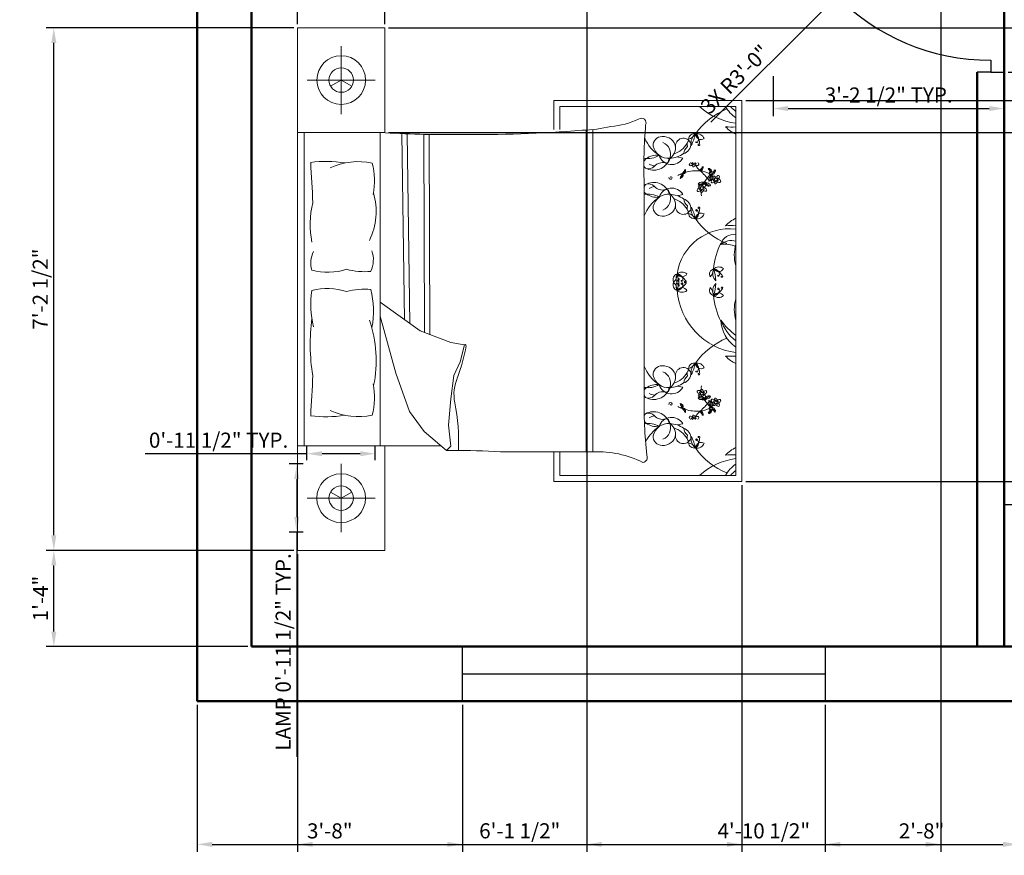
# Model space of a CAD drawing. Units: inches. Extents: x 3242 to 3618, y 1365 to 1814.
# Tile 1 of 6: x 3242 to 3405, y 1376 to 1514. Entities that reach past the tile are written whole.
import ezdxf

# ---------------------------------------------------------------- set-up
doc = ezdxf.new("R2010")
doc.units = ezdxf.units.IN
for name, color, linetype, lineweight in [('A-ANNO-DIMS', 2, 'Continuous', 18), ('A-DOOR', 4, 'Continuous', 25), ('A-FLOR-CASE', 8, 'Continuous', 25), ('A-FURN', 8, 'Continuous', 18), ('A-GLAZ', 5, 'Continuous', 25), ('A-WALL', 7, 'Continuous', 50)]:
    doc.layers.add(name, color=color, linetype=linetype, lineweight=lineweight)
doc.styles.get("Standard").update_dxf_attribs({"font": 'arial.ttf'})
doc.dimstyles.new('ISO-25', dxfattribs={"dimtxt": 2.5, "dimasz": 2.5, "dimexe": 1.25, "dimexo": 0.625, "dimtad": 1, "dimdec": 0, "dimlunit": 3, "dimtxsty": 'Standard', "dimcen": 2.5, "dimadec": 0, "dimazin": 0, "dimtfac": 1, "dimtdec": 0, "dimtmove": 0, "dimatfit": 3, "dimfxl": 1, "dimarcsym": 0})

# ---------------------------------------------------------------- blocks, each defined once
blk = doc.blocks.new('DOOR-SWING-36IN')
for p, q in [((33.75, 40), (38.25, 40)), ((36, 40), (36, 38)), ((36, 38), (0, 38)), ((38.25, 37), (0, 37)), ((36, 2), (36, 0)), ((36, 0), (33.75, 0)), ((36, 0), (38.25, 0))]:
    blk.add_line(p, q)
blk.add_arc((36, 38), 36, 180, 270)
blk = doc.blocks.new('WINDOW-60IN')
for p, q in [((0, 9), (60, 9)), ((0, 0), (0, 9)), ((60, 9), (60, 0)), ((0, 4.5), (60, 4.5)), ((60, 0), (0, 0))]:
    blk.add_line(p, q)
blk = doc.blocks.new('BEDSIDE-LAMP-LG')
for p, q in [((5.65, 0), (5.65, 11.29)), ((11.29, 5.65), (0, 5.65))]:
    blk.add_line(p, q)
for points in [[(5.65, 5.65), (3.9, 4.64)], [(5.65, 5.65), (7.39, 4.64)]]:
    blk.add_lwpolyline(points)
for radius in [4.03, 2.02]:
    blk.add_circle((5.65, 5.65), radius)
blk = doc.blocks.new('*D17')
at = {"layer": 'A-ANNO-DIMS', "color": 0, "lineweight": -2, "transparency": 16777216}
for p, q in [((3405.61, 1545.66), (3412.23, 1545.66)), ((3410.98, 1508.16), (3410.98, 1543.16)), ((3405.61, 1505.66), (3412.23, 1505.66))]:
    blk.add_line(p, q, dxfattribs=at)
at = {"layer": 'A-ANNO-DIMS', "color": 0, "transparency": 16777216}
for points in [[(3410.56, 1543.16), (3411.4, 1543.16), (3410.98, 1545.66)], [(3410.56, 1508.16), (3411.4, 1508.16), (3410.98, 1505.66)]]:
    blk.add_solid(points, dxfattribs=at)
at = {"layer": 'Defpoints', "color": 0, "transparency": 16777216}
for p in [(3404.98, 1545.66), (3410.98, 1545.66), (3404.98, 1505.66)]:
    blk.add_point(p, dxfattribs=at)
at = {"layer": 'A-ANNO-DIMS', "color": 0, "transparency": 16777216, "insert": (3409.06, 1525.66), "char_height": 2.5, "attachment_point": 5, "rotation": 90}
blk.add_mtext('DOOR 3\'-4" TYP.', dxfattribs=at)
blk = doc.blocks.new('*D18')
at = {"layer": 'A-ANNO-DIMS', "color": 0, "lineweight": -2, "transparency": 16777216}
for p, q in [((3366.73, 1505.03), (3366.73, 1498.41)), ((3404.98, 1505.03), (3404.98, 1498.41)), ((3369.23, 1499.66), (3402.48, 1499.66))]:
    blk.add_line(p, q, dxfattribs=at)
at = {"layer": 'A-ANNO-DIMS', "color": 0, "transparency": 16777216}
for points in [[(3369.23, 1500.07), (3369.23, 1499.24), (3366.73, 1499.66)], [(3402.48, 1500.07), (3402.48, 1499.24), (3404.98, 1499.66)]]:
    blk.add_solid(points, dxfattribs=at)
at = {"layer": 'Defpoints', "color": 0, "transparency": 16777216}
for p in [(3366.73, 1505.66), (3404.98, 1505.66), (3404.98, 1499.66)]:
    blk.add_point(p, dxfattribs=at)
at = {"layer": 'A-ANNO-DIMS', "color": 0, "transparency": 16777216, "insert": (3385.86, 1501.57), "char_height": 2.5, "attachment_point": 5}
blk.add_mtext('3\'-2 1/2" TYP.', dxfattribs=at)
blk = doc.blocks.new('*D31')
at = {"layer": 'A-ANNO-DIMS', "color": 0, "lineweight": -2, "transparency": 16777216}
for p, q in [((3289.03, 1440.87), (3286.71, 1440.87)), ((3287.96, 1438.37), (3287.96, 1432.08)), ((3289.03, 1429.58), (3286.71, 1429.58)), ((3287.96, 1429.58), (3287.96, 1392.45))]:
    blk.add_line(p, q, dxfattribs=at)
at = {"layer": 'A-ANNO-DIMS', "color": 0, "transparency": 16777216}
for points in [[(3287.54, 1438.37), (3288.38, 1438.37), (3287.96, 1440.87)], [(3287.54, 1432.08), (3288.38, 1432.08), (3287.96, 1429.58)]]:
    blk.add_solid(points, dxfattribs=at)
at = {"layer": 'Defpoints', "color": 0, "transparency": 16777216}
for p in [(3289.65, 1440.87), (3287.96, 1429.58), (3289.65, 1429.58)]:
    blk.add_point(p, dxfattribs=at)
at = {"layer": 'A-ANNO-DIMS', "color": 0, "transparency": 16777216, "insert": (3286.04, 1409.77), "char_height": 2.5, "attachment_point": 5, "rotation": 90}
blk.add_mtext('LAMP 0\'-11 1/2" TYP.', dxfattribs=at)
blk = doc.blocks.new('*D32')
at = {"layer": 'A-ANNO-DIMS', "color": 0, "lineweight": -2, "transparency": 16777216}
for p, q in [((3289.65, 1441.5), (3289.65, 1443.81)), ((3300.95, 1441.5), (3300.95, 1443.81)), ((3289.65, 1442.56), (3262.9, 1442.56)), ((3298.45, 1442.56), (3292.15, 1442.56))]:
    blk.add_line(p, q, dxfattribs=at)
at = {"layer": 'A-ANNO-DIMS', "color": 0, "transparency": 16777216}
for points in [[(3292.15, 1442.98), (3292.15, 1442.15), (3289.65, 1442.56)], [(3298.45, 1442.98), (3298.45, 1442.15), (3300.95, 1442.56)]]:
    blk.add_solid(points, dxfattribs=at)
at = {"layer": 'Defpoints', "color": 0, "transparency": 16777216}
for p in [(3289.65, 1442.56), (3289.65, 1440.87), (3300.95, 1440.87)]:
    blk.add_point(p, dxfattribs=at)
at = {"layer": 'A-ANNO-DIMS', "color": 0, "transparency": 16777216, "insert": (3275.03, 1444.48), "char_height": 2.5, "attachment_point": 5}
blk.add_mtext('0\'-11 1/2" TYP.', dxfattribs=at)
blk = doc.blocks.new('*D39')
at = {"layer": 'A-ANNO-DIMS', "color": 0, "lineweight": -2, "transparency": 16777216}
for p, q in [((3271.48, 1401.03), (3271.48, 1376.71)), ((3315.35, 1401.03), (3315.35, 1376.71)), ((3273.98, 1377.96), (3312.85, 1377.96))]:
    blk.add_line(p, q, dxfattribs=at)
at = {"layer": 'A-ANNO-DIMS', "color": 0, "transparency": 16777216}
for points in [[(3273.98, 1378.37), (3273.98, 1377.54), (3271.48, 1377.96)], [(3312.85, 1378.37), (3312.85, 1377.54), (3315.35, 1377.96)]]:
    blk.add_solid(points, dxfattribs=at)
at = {"layer": 'Defpoints', "color": 0, "transparency": 16777216}
for p in [(3271.48, 1401.66), (3315.35, 1401.66), (3315.35, 1377.96)]:
    blk.add_point(p, dxfattribs=at)
at = {"layer": 'A-ANNO-DIMS', "color": 0, "transparency": 16777216, "insert": (3293.42, 1379.86), "char_height": 2.5, "attachment_point": 5}
blk.add_mtext('3\'-8"', dxfattribs=at)
blk = doc.blocks.new('*D40')
at = {"layer": 'A-ANNO-DIMS', "color": 0, "lineweight": -2, "transparency": 16777216}
for p, q in [((3375.35, 1401.03), (3375.35, 1376.71)), ((3407.26, 1401.03), (3407.26, 1376.71)), ((3377.85, 1377.96), (3404.76, 1377.96))]:
    blk.add_line(p, q, dxfattribs=at)
at = {"layer": 'A-ANNO-DIMS', "color": 0, "transparency": 16777216}
for points in [[(3377.85, 1378.37), (3377.85, 1377.54), (3375.35, 1377.96)], [(3404.76, 1378.37), (3404.76, 1377.54), (3407.26, 1377.96)]]:
    blk.add_solid(points, dxfattribs=at)
at = {"layer": 'Defpoints', "color": 0, "transparency": 16777216}
for p in [(3375.35, 1401.66), (3407.26, 1401.66), (3407.26, 1377.96)]:
    blk.add_point(p, dxfattribs=at)
at = {"layer": 'A-ANNO-DIMS', "color": 0, "transparency": 16777216, "insert": (3391.3, 1379.86), "char_height": 2.5, "attachment_point": 5}
blk.add_mtext('2\'-8"', dxfattribs=at)
blk = doc.blocks.new('*D48')
at = {"layer": 'A-ANNO-DIMS', "color": 0, "lineweight": -2, "transparency": 16777216}
for p, q in [((3394.48, 1651.75), (3394.48, 1376.71)), ((3335.91, 1642.66), (3335.91, 1376.71)), ((3338.41, 1377.96), (3391.98, 1377.96))]:
    blk.add_line(p, q, dxfattribs=at)
at = {"layer": 'A-ANNO-DIMS', "color": 0, "transparency": 16777216}
for points in [[(3338.41, 1378.37), (3338.41, 1377.54), (3335.91, 1377.96)], [(3391.98, 1378.37), (3391.98, 1377.54), (3394.48, 1377.96)]]:
    blk.add_solid(points, dxfattribs=at)
at = {"layer": 'Defpoints', "color": 0, "transparency": 16777216}
for p in [(3394.48, 1652.37), (3335.91, 1643.28), (3394.48, 1377.96)]:
    blk.add_point(p, dxfattribs=at)
at = {"layer": 'A-ANNO-DIMS', "color": 0, "transparency": 16777216, "insert": (3365.2, 1379.87), "char_height": 2.5, "attachment_point": 5}
blk.add_mtext('4\'-10 1/2"', dxfattribs=at)
blk = doc.blocks.new('*D53')
at = {"layer": 'A-ANNO-DIMS', "color": 0, "lineweight": -2, "transparency": 16777216}
for p, q in [((3361.59, 1437.36), (3361.59, 1376.71)), ((3288.1, 1425.96), (3288.1, 1376.71)), ((3290.6, 1377.96), (3359.09, 1377.96))]:
    blk.add_line(p, q, dxfattribs=at)
at = {"layer": 'A-ANNO-DIMS', "color": 0, "transparency": 16777216}
for points in [[(3290.6, 1378.37), (3290.6, 1377.54), (3288.1, 1377.96)], [(3359.09, 1378.37), (3359.09, 1377.54), (3361.59, 1377.96)]]:
    blk.add_solid(points, dxfattribs=at)
at = {"layer": 'Defpoints', "color": 0, "transparency": 16777216}
for p in [(3361.59, 1437.99), (3288.1, 1426.58), (3361.59, 1377.96)]:
    blk.add_point(p, dxfattribs=at)
at = {"layer": 'A-ANNO-DIMS', "color": 0, "transparency": 16777216, "insert": (3324.84, 1379.87), "char_height": 2.5, "attachment_point": 5}
blk.add_mtext('6\'-1 1/2"', dxfattribs=at)
blk = doc.blocks.new('*D54')
at = {"layer": 'A-ANNO-DIMS', "color": 0, "lineweight": -2, "transparency": 16777216}
for p, q in [((3362.21, 1500.99), (3617.43, 1500.99)), ((3616.18, 1440.49), (3616.18, 1498.49)), ((3362.21, 1437.99), (3617.43, 1437.99))]:
    blk.add_line(p, q, dxfattribs=at)
at = {"layer": 'A-ANNO-DIMS', "color": 0, "transparency": 16777216}
for points in [[(3615.76, 1498.49), (3616.6, 1498.49), (3616.18, 1500.99)], [(3615.76, 1440.49), (3616.6, 1440.49), (3616.18, 1437.99)]]:
    blk.add_solid(points, dxfattribs=at)
at = {"layer": 'Defpoints', "color": 0, "transparency": 16777216}
for p in [(3361.59, 1500.99), (3616.18, 1500.99), (3361.59, 1437.99)]:
    blk.add_point(p, dxfattribs=at)
at = {"layer": 'A-ANNO-DIMS', "color": 0, "transparency": 16777216, "insert": (3614.28, 1469.49), "char_height": 2.5, "attachment_point": 5, "rotation": 90}
blk.add_mtext('5\'-3"', dxfattribs=at)
blk = doc.blocks.new('*D55')
at = {"layer": 'A-ANNO-DIMS', "color": 0, "lineweight": -2, "transparency": 16777216}
for p, q in [((3303.13, 1513), (3617.43, 1513)), ((3616.18, 1510.5), (3616.18, 1498.21)), ((3303.13, 1495.71), (3617.43, 1495.71))]:
    blk.add_line(p, q, dxfattribs=at)
at = {"layer": 'A-ANNO-DIMS', "color": 0, "transparency": 16777216}
for points in [[(3615.76, 1510.5), (3616.6, 1510.5), (3616.18, 1513)], [(3615.76, 1498.21), (3616.6, 1498.21), (3616.18, 1495.71)]]:
    blk.add_solid(points, dxfattribs=at)
at = {"layer": 'Defpoints', "color": 0, "transparency": 16777216}
for p in [(3302.5, 1513), (3302.5, 1495.71), (3616.18, 1495.71)]:
    blk.add_point(p, dxfattribs=at)
at = {"layer": 'A-ANNO-DIMS', "color": 0, "transparency": 16777216, "insert": (3614.26, 1504.35), "char_height": 2.5, "attachment_point": 5, "rotation": 90}
blk.add_mtext('1\'-5 1/2"', dxfattribs=at)
blk = doc.blocks.new('*D56')
at = {"layer": 'A-ANNO-DIMS', "color": 0, "lineweight": -2, "transparency": 16777216}
for p, q in [((3288.1, 1513.62), (3288.1, 1783.61)), ((3302.5, 1513.62), (3302.5, 1783.61)), ((3290.6, 1782.36), (3300, 1782.36))]:
    blk.add_line(p, q, dxfattribs=at)
at = {"layer": 'A-ANNO-DIMS', "color": 0, "transparency": 16777216}
for points in [[(3290.6, 1782.77), (3290.6, 1781.94), (3288.1, 1782.36)], [(3300, 1782.77), (3300, 1781.94), (3302.5, 1782.36)]]:
    blk.add_solid(points, dxfattribs=at)
at = {"layer": 'Defpoints', "color": 0, "transparency": 16777216}
for p in [(3302.5, 1782.36), (3288.1, 1513), (3302.5, 1513)]:
    blk.add_point(p, dxfattribs=at)
at = {"layer": 'A-ANNO-DIMS', "color": 0, "transparency": 16777216, "insert": (3295.3, 1784.27), "char_height": 2.5, "attachment_point": 5}
blk.add_mtext('1\'-2 1/2"', dxfattribs=at)
blk = doc.blocks.new('*D57')
at = {"layer": 'A-ANNO-DIMS', "color": 0, "lineweight": -2, "transparency": 16777216}
for p, q in [((3287.47, 1513), (3246.53, 1513)), ((3247.78, 1429.08), (3247.78, 1510.5)), ((3287.47, 1426.58), (3246.53, 1426.58))]:
    blk.add_line(p, q, dxfattribs=at)
at = {"layer": 'A-ANNO-DIMS', "color": 0, "transparency": 16777216}
for points in [[(3247.36, 1510.5), (3248.2, 1510.5), (3247.78, 1513)], [(3247.36, 1429.08), (3248.2, 1429.08), (3247.78, 1426.58)]]:
    blk.add_solid(points, dxfattribs=at)
at = {"layer": 'Defpoints', "color": 0, "transparency": 16777216}
for p in [(3247.78, 1513), (3288.1, 1513), (3288.1, 1426.58)]:
    blk.add_point(p, dxfattribs=at)
at = {"layer": 'A-ANNO-DIMS', "color": 0, "transparency": 16777216, "insert": (3245.86, 1469.79), "char_height": 2.5, "attachment_point": 5, "rotation": 90}
blk.add_mtext('7\'-2 1/2"', dxfattribs=at)
blk = doc.blocks.new('*D59')
at = {"layer": 'A-ANNO-DIMS', "color": 0, "lineweight": -2, "transparency": 16777216}
for p, q in [((3287.47, 1426.58), (3246.53, 1426.58)), ((3247.78, 1413.16), (3247.78, 1424.08)), ((3279.86, 1410.66), (3246.53, 1410.66))]:
    blk.add_line(p, q, dxfattribs=at)
at = {"layer": 'A-ANNO-DIMS', "color": 0, "transparency": 16777216}
for points in [[(3247.36, 1424.08), (3248.2, 1424.08), (3247.78, 1426.58)], [(3247.36, 1413.16), (3248.2, 1413.16), (3247.78, 1410.66)]]:
    blk.add_solid(points, dxfattribs=at)
at = {"layer": 'Defpoints', "color": 0, "transparency": 16777216}
for p in [(3247.78, 1426.58), (3288.1, 1426.58), (3280.48, 1410.66)]:
    blk.add_point(p, dxfattribs=at)
at = {"layer": 'A-ANNO-DIMS', "color": 0, "transparency": 16777216, "insert": (3245.9, 1418.62), "char_height": 2.5, "attachment_point": 5, "rotation": 90}
blk.add_mtext('1\'-4"', dxfattribs=at)
blk = doc.blocks.new('*D65')
at = {"layer": 'A-ANNO-DIMS', "color": 0, "lineweight": -2, "transparency": 16777216}
for p, q in [((3402.73, 1543.66), (3377.27, 1518.2)), ((3356.46, 1497.39), (3375.51, 1516.43))]:
    blk.add_line(p, q, dxfattribs=at)
at = {"layer": 'A-ANNO-DIMS', "color": 0, "transparency": 16777216}
blk.add_solid([(3375.21, 1516.73), (3375.8, 1516.14), (3377.27, 1518.2)], dxfattribs=at)
at = {"layer": 'Defpoints', "color": 0, "transparency": 16777216}
for p in [(3402.73, 1543.66), (3377.27, 1518.2)]:
    blk.add_point(p, dxfattribs=at)
at = {"layer": 'A-ANNO-DIMS', "color": 0, "transparency": 16777216, "insert": (3360.66, 1504.27), "char_height": 2.5, "attachment_point": 5, "rotation": 44.9992}
blk.add_mtext('3X R3\'-0"', dxfattribs=at)

msp = doc.modelspace()

# ---------------------------------------------------------------- linework, layer by layer
at = {"layer": 'A-FLOR-CASE'}
msp.add_line((3483.26, 1434.12), (3404.98, 1434.12), dxfattribs=at)
at = {"layer": 'A-FURN'}
for p, q in [((3288.1, 1426.58), (3288.1, 1513)), ((3330.46, 1496.2), (3330.46, 1500.99)), ((3330.46, 1500.99), (3361.59, 1500.99)), ((3331.46, 1499.99), (3331.46, 1496.18)), ((3360.59, 1499.99), (3331.46, 1499.99)), ((3360.59, 1438.99), (3360.59, 1499.99)), ((3361.59, 1500.99), (3361.59, 1437.99)), ((3289.21, 1495.71), (3289.21, 1443.87)), ((3301.75, 1443.87), (3301.75, 1495.71)), ((3305.34, 1495.48), (3305.78, 1464.72)), ((3306.23, 1495.45), (3306.67, 1464.07)), ((3308.95, 1495.4), (3309.08, 1462.59)), ((3309.84, 1495.41), (3309.98, 1462.25)), ((3335.85, 1496.11), (3335.85, 1442.87)), ((3336.93, 1496.19), (3336.93, 1442.87)), ((3351.82, 1491.47), (3350.85, 1491.66)), ((3345.41, 1487.33), (3345.41, 1452.25)), ((3351.82, 1485.43), (3350.85, 1485.24)), ((3301.75, 1467.61), (3308.35, 1462.87)), ((3304.32, 1455.87), (3301.75, 1465.29)), ((3308.35, 1462.87), (3313.42, 1460.94)), ((3313.42, 1460.94), (3315.69, 1460.59)), ((3315.69, 1460.59), (3314.99, 1457.79)), ((3314.99, 1457.79), (3313.94, 1455.52)), ((3306.6, 1449.57), (3304.32, 1455.87)), ((3313.94, 1455.52), (3313.42, 1451.67)), ((3351.82, 1453.55), (3350.85, 1453.74)), ((3313.42, 1451.67), (3313.07, 1447.29)), ((3309.05, 1446.24), (3306.6, 1449.57)), ((3312.72, 1443.09), (3309.05, 1446.24)), ((3313.07, 1447.29), (3313.42, 1443.79)), ((3351.82, 1447.51), (3350.85, 1447.32)), ((3288.1, 1443.87), (3311.82, 1443.87)), ((3313.42, 1443.79), (3312.72, 1443.09)), ((3330.46, 1437.99), (3330.46, 1442.88)), ((3331.46, 1442.88), (3331.46, 1438.99)), ((3361.59, 1437.99), (3330.46, 1437.99)), ((3331.46, 1438.99), (3360.59, 1438.99))]:
    msp.add_line(p, q, dxfattribs=at)
for points in [[(3288.1, 1495.71), (3302.5, 1495.71), (3302.5, 1513), (3288.1, 1513)], [(3302.5, 1443.87), (3302.5, 1426.58), (3288.1, 1426.58)]]:
    msp.add_lwpolyline(points, dxfattribs=at)
for points in [[(3335.17, 1496.08, 0.056112), (3339.92, 1496.71, 0.095341), (3344.5, 1497.92)], [(3290.25, 1490.75, -0.074897), (3295.9, 1490.65, 0.472817)], [(3296.21, 1473.08, -0.14099), (3290.45, 1472.9, -0.235245)], [(3296.21, 1469.38, 0.14099), (3290.45, 1469.56, 0.235245)], [(3290.25, 1448.83, 0.074897), (3295.9, 1448.93, -0.472817)], [(3320.63, 1442.91, 0.001242), (3337.03, 1442.87, -0.127202), (3345.2, 1441.14)]]:
    msp.add_lwpolyline(points, format="xyb", dxfattribs=at)
for centre in [(3357.28, 1487.92), (3354.96, 1486.48), (3354.96, 1452.5), (3357.28, 1451.06)]:
    msp.add_circle(centre, 0.22, dxfattribs=at)
for centre, radius, start, end in [((3362.11, 1508.39), 11.28, 228.1144, 262.255), ((3363.62, 1502.73), 5.5, 209.8884, 236.5383), ((3364.64, 1504.7), 6.85, 223.5186, 233.6964), ((3363.22, 1489.08), 11.28, 111.4092, 145.6135), ((3344.94, 1497.27), 0.788, 336.5219, 123.8264), ((3429.46, 1489.98), 84.09, 175.2402, 181.8035), ((3362.35, 1499.65), 4.59, 221.0454, 247.4453), ((3359.88, 1512.21), 15.61, 266.3481, 272.5919), ((3312.32, 1650.62), 155.27, 266.1, 270.9282), ((3317.96, 1697.89), 202.54, 269.1145, 274.8735), ((3348.36, 1493.57), 1.46, 88.9462, 185.5144), ((3348.57, 1492.97), 2.06, 7.1143, 95.0551), ((3353.69, 1494.55), 0.935, 76.272, 177.0484), ((3352.26, 1496.46), 1.93, 284.7031, 328.6173), ((3354.95, 1494.01), 1.78, 125.7657, 194.5347), ((3346.2, 1497.17), 7.89, 332.8176, 347.4827), ((3354.18, 1494.23), 1.25, 20.9613, 102.2885), ((3354.85, 1495.48), 0.942, 181.7131, 301.5367), ((3351.76, 1493.58), 2.85, 2.0648, 41.1598), ((3353.48, 1494.64), 0.923, 316.2238, 62.3173), ((3351.5, 1497.38), 6.54, 203.6453, 236.3329), ((3349.44, 1494.02), 2.6, 193.079, 274.7067), ((3347.78, 1492.16), 2.01, 338.5779, 68.4181), ((3349.04, 1496.02), 4.08, 288.2955, 328.7386), ((3351.89, 1493.45), 1.3, 19.1312, 189.736), ((3351.5, 1493.76), 1.62, 285.6955, 4.031), ((3353.66, 1492.01), 1.72, 128.4175, 173.8338), ((3353.3, 1493.71), 0.795, 126.7319, 206.0245), ((3354.01, 1494.1), 0.0736, 20.2667, 316.2271), ((3354.47, 1493.67), 0.14, 168.5166, 2.0648), ((3354.4, 1493.69), 0.0681, 52.0591, 168.5166), ((3346.05, 1494.98), 3.58, 259.249, 301.1782), ((3347.61, 1488.62), 3.33, 85.2696, 124.215), ((3349.96, 1492.54), 2.15, 196.8663, 330.0915), ((3348.11, 1493.33), 2.51, 305.9599, 357.6409), ((3349.37, 1496.06), 4.64, 273.4924, 303.7117), ((2467.9, 1443.12), 823.74, 2.85022, 3.31479), ((3298.16, 1479.74), 11.14, 78.2417, 114.8684), ((3289.24, 1487.67), 11.58, 348.9631, 14.8961), ((3346.37, 1490.55), 1.04, 196.6343, 225.5483), ((3346.37, 1490.55), 1.04, 127.675, 162.5814), ((3346.98, 1492.21), 2.75, 240.8249, 340.7178), ((3346.16, 1490.99), 1.29, 246.1646, 318.4347), ((3347.48, 1492.62), 2.48, 240.0851, 262.564), ((3348.46, 1488.95), 1.77, 74.8529, 138.4347), ((3349.06, 1491.18), 0.536, 254.8529, 12.6959), ((3347.61, 1488.62), 3.33, 53.6555, 57.2989), ((3353.05, 1490.37), 0.17, 125.0752, 284.7644), ((3353.31, 1490.44), 0.367, 127.3642, 168.4363), ((3353.02, 1490.73), 0.529, 277.4968, 341.2737), ((3353.44, 1490.49), 0.21, 88.1325, 178.8919), ((3353.86, 1490.26), 0.455, 136.3462, 189.6513), ((3353.6, 1490.22), 0.19, 189.6513, 312.3208), ((3353.65, 1490.74), 0.22, 183.2768, 356.7232), ((3354.34, 1490.35), 0.72, 164.2829, 186.9148), ((3353.49, 1490.35), 0.36, 312.3208, 40.2111), ((3354.25, 1490.75), 0.511, 201.6382, 274.947), ((3353.57, 1490.05), 0.668, 42.3896, 66.5724), ((3360.31, 1495.34), 8.2, 217.9541, 226.8459), ((3354.06, 1490.44), 0.363, 10.9597, 52.2379), ((3354.28, 1490.41), 0.169, 274.947, 37.5263), ((3355.35, 1489.67), 0.454, 115.5379, 168.6744), ((3353.82, 1490.32), 1.37, 329.344, 349.7412), ((3352.72, 1490.01), 2.44, 352.8698, 1.6736), ((3354.22, 1482.21), 7.16, 110.1059, 116.9968), ((3351.82, 1488.11), 0.454, 129.5056, 182.6421), ((3350.52, 1489.16), 1.37, 308.4388, 328.836), ((3350.26, 1489.02), 1.39, 336.3901, 344.4871), ((3351.77, 1488.66), 0.176, 83.9457, 185.6216), ((3351.07, 1488.83), 0.724, 328.836, 0.8141), ((3351.44, 1488.62), 0.415, 306.5232, 32.4668), ((3351.94, 1488.94), 0.176, 112.5583, 214.2343), ((3351.82, 1489.25), 0.415, 265.7131, 351.6568), ((3351.46, 1489.48), 0.724, 297.3659, 329.344), ((3350.91, 1490.11), 1.39, 313.6929, 321.7899), ((3352.45, 1489.16), 0.454, 115.5379, 168.6744), ((3350.91, 1489.81), 1.37, 329.344, 349.7412), ((3354.22, 1482.21), 7.16, 86.1723, 106.4158), ((3349.82, 1489.5), 2.44, 352.8698, 1.6736), ((3354.85, 1489.45), 0.176, 112.5583, 214.2343), ((3354.73, 1489.77), 0.415, 265.7131, 351.6568), ((3354.37, 1490), 0.724, 297.3659, 329.344), ((3354.4, 1485.78), 3.59, 60.7959, 85.244), ((3346.76, 1480.61), 11.81, 37.8256, 47.7588), ((3353.82, 1490.62), 1.39, 313.6929, 321.7899), ((3359.17, 1485.41), 4.3, 130.182, 149.456), ((3356.15, 1489.52), 0.246, 33.0979, 123.1364), ((3350.74, 1486.05), 6.43, 31.1156, 34.8118), ((3355.79, 1489.1), 0.665, 2.3172, 70.5201), ((3355.47, 1488.38), 1, 310.9365, 22.7695), ((3356.34, 1488.93), 0.192, 135.7354, 318.1297), ((3356.02, 1489.25), 0.254, 315.7354, 31.1156), ((3355.81, 1488.71), 0.59, 319.3812, 5.5456), ((3356.49, 1488.93), 0.192, 68.2452, 250.6395), ((3356.05, 1489.17), 0.573, 352.6008, 57.1845), ((3358.09, 1485.33), 3.83, 111.7087, 116.2181), ((3354.4, 1485.78), 3.59, 47.5083, 55.9967), ((3356.59, 1489.3), 0.573, 252.8042, 349.6943), ((3356.05, 1488.28), 0.61, 331.1838, 51.6792), ((3356.65, 1489.35), 0.254, 248.2452, 323.6254), ((3356.43, 1489.5), 0.665, 291.7087, 3.0299), ((3356.97, 1488.16), 0.3, 358.5719, 143.8954), ((3351.68, 1493.01), 6.43, 323.6254, 327.3216), ((3356.95, 1489.34), 0.246, 325.6077, 55.6462), ((3357.94, 1487.98), 0.694, 121.9501, 165.2442), ((3357.44, 1488.37), 0.434, 278.5614, 22.5914), ((3357.69, 1488.38), 0.218, 44.3732, 121.9501), ((3346.37, 1486.35), 1.04, 134.4517, 156.7144), ((3346.98, 1484.69), 2.75, 19.2822, 119.1751), ((3346.16, 1485.91), 1.29, 41.5653, 113.8354), ((3349.77, 1488.22), 0.271, 169.5864, 349.5616), ((3349.87, 1488.2), 0.167, 349.5616, 167.2949), ((3350.28, 1490.27), 2.44, 296.5064, 305.3102), ((3354.63, 1488.16), 1, 253.6301, 325.4631), ((3354.91, 1486.77), 0.71, 82.0748, 142.6895), ((3354.83, 1487.75), 0.729, 228.342, 274.9894), ((3354.57, 1486.75), 0.216, 138.2946, 276.2474), ((3354.65, 1486.72), 0.3, 358.5719, 143.8954), ((3354.82, 1486.96), 0.303, 208.8493, 269.9355), ((3354.85, 1487.63), 0.61, 273.8774, 357.1501), ((3355.62, 1486.54), 0.694, 121.9501, 165.2442), ((3355.09, 1488.06), 0.59, 262.0748, 308.2393), ((3355.14, 1486.8), 0.146, 262.868, 7.094), ((3355.12, 1486.93), 0.434, 278.5614, 22.5914), ((3359.17, 1485.41), 4.3, 156.1523, 156.9499), ((3355.37, 1486.94), 0.218, 44.3732, 121.9501), ((3356.04, 1487.45), 0.61, 181.4625, 249.4747), ((3355.94, 1487.93), 0.59, 215.1128, 261.2773), ((3356.41, 1487.9), 1, 197.889, 269.722), ((3356.1, 1487.56), 0.729, 248.3627, 295.0101), ((3355.74, 1486.65), 0.71, 20.6625, 81.2773), ((3356.8, 1487.86), 0.71, 139.3812, 199.9959), ((3355.94, 1488.32), 0.729, 285.6484, 332.2957), ((3356.67, 1487.55), 0.17, 125.0752, 284.7644), ((3356.93, 1487.61), 0.367, 93.635, 168.4363), ((3356.89, 1488.19), 0.216, 138.2946, 276.2474), ((3356.65, 1487.91), 0.529, 277.4968, 341.2737), ((3357.07, 1487.66), 0.21, 88.1325, 178.8919), ((3357.14, 1488.4), 0.303, 208.8493, 269.9355), ((3356.89, 1488.32), 0.346, 274.2123, 318.1587), ((3357.49, 1487.44), 0.455, 136.3462, 189.6513), ((3357.23, 1487.39), 0.19, 189.6513, 312.3208), ((3357.96, 1487.52), 0.72, 164.2829, 186.9148), ((3357.11, 1487.52), 0.36, 312.3208, 40.2111), ((3357.88, 1487.93), 0.511, 201.6382, 274.947), ((3357.46, 1488.24), 0.146, 262.868, 7.094), ((3357.2, 1487.23), 0.668, 42.3896, 66.5724), ((3357.68, 1487.62), 0.363, 10.9597, 118.7804), ((3357.91, 1487.58), 0.169, 274.947, 37.5263), ((3290.09, 1482.67), 11, 333.8761, 16.1746), ((3346.37, 1486.35), 1.04, 203.2856, 232.325), ((3346.05, 1481.92), 3.58, 58.8218, 100.2867), ((3347.61, 1488.29), 3.33, 235.785, 274.7304), ((3347.48, 1484.28), 2.48, 97.436, 119.9149), ((3349.44, 1482.88), 2.6, 85.2933, 166.921), ((3348.46, 1487.95), 1.77, 221.5653, 285.1471), ((3349.96, 1484.36), 2.15, 29.9085, 163.1337), ((3347.78, 1484.74), 2.01, 291.5819, 21.4221), ((3349.06, 1485.72), 0.536, 347.3041, 105.1471), ((3347.61, 1488.29), 3.33, 302.7011, 306.3445), ((3348.11, 1483.57), 2.51, 2.3591, 54.0401), ((3349.37, 1480.85), 4.64, 56.2883, 86.5076), ((3354.35, 1486.11), 0.17, 125.0752, 284.7644), ((3354.61, 1486.17), 0.367, 93.635, 168.4363), ((3354.33, 1486.47), 0.529, 277.4968, 341.2737), ((3354.75, 1486.22), 0.21, 88.1325, 178.8919), ((3354.57, 1486.89), 0.346, 274.2123, 318.1587), ((3355.17, 1486), 0.455, 136.3462, 189.6513), ((3354.91, 1485.95), 0.19, 189.6513, 312.3208), ((3359.17, 1485.41), 4.3, 175.2415, 182.8929), ((3355.64, 1486.08), 0.72, 164.2829, 186.9148), ((3354.79, 1486.08), 0.36, 312.3208, 40.2111), ((3355.56, 1486.49), 0.511, 201.6382, 274.947), ((3354.88, 1485.79), 0.668, 42.3896, 66.5724), ((3355.36, 1486.18), 0.363, 10.9597, 118.7804), ((3355.59, 1486.14), 0.169, 274.947, 37.5263), ((3305.37, 1480.49), 15.19, 166.3427, 191.1841), ((3351.5, 1479.52), 6.54, 123.6671, 158.5059), ((3348.57, 1483.93), 2.06, 264.9449, 352.8857), ((3349.04, 1480.88), 4.08, 31.2614, 71.7045), ((3351.89, 1483.45), 1.3, 170.264, 340.8688), ((3353.66, 1484.89), 1.72, 186.1662, 231.5825), ((3351.5, 1483.14), 1.62, 355.969, 74.3045), ((3353.3, 1483.19), 0.795, 153.9755, 233.2681), ((3348.36, 1483.33), 1.46, 174.4856, 271.0538), ((3353.69, 1482.36), 0.935, 182.9516, 283.728), ((3352.26, 1480.44), 1.93, 31.3827, 75.2969), ((3354.95, 1482.9), 1.78, 165.4653, 234.2343), ((3346.2, 1479.74), 7.89, 12.5173, 27.1824), ((3351.76, 1483.33), 2.85, 318.8402, 357.9352), ((3353.48, 1482.26), 0.923, 297.6827, 43.7762), ((3354.85, 1481.42), 0.942, 58.4633, 178.2869), ((3354.18, 1482.67), 1.25, 257.7115, 339.0387), ((3354.06, 1482.82), 0.122, 43.7762, 339.7183), ((3354.47, 1483.23), 0.14, 357.9352, 191.4834), ((3354.4, 1483.21), 0.0681, 191.4834, 307.9409), ((3363.22, 1487.82), 11.28, 214.3865, 248.5908), ((3362.35, 1477.26), 4.59, 112.5547, 138.9546), ((3359.88, 1464.69), 15.61, 87.4081, 93.6519), ((3359.5, 1471.03), 8.73, 82.8636, 171.8197), ((3360.11, 1476.79), 2.03, 76.3898, 169.0739), ((3368.15, 1472.26), 11.28, 152.5854, 175.5377), ((3359.83, 1475.27), 2.56, 72.8609, 131.9049), ((3358.7, 1472.16), 5.05, 68.117, 96.6195), ((3366.52, 1475.42), 6.2, 162.9798, 196.4569), ((3294.56, 1474.09), 4.27, 153.3437, 196.1026), ((3296.05, 1474.67), 4.58, 335.0183, 18.5407), ((3369.72, 1472.96), 9.18, 174.3643, 175.6213), ((3299.1, 1483.26), 10.59, 254.1707, 275.9871), ((3351.12, 1471.38), 0.935, 106.1963, 206.9726), ((3348.93, 1472.32), 1.93, 314.6273, 358.5415), ((3352.48, 1471.54), 1.78, 155.6899, 224.4589), ((3351.7, 1471.35), 1.25, 50.8855, 132.2127), ((3351.66, 1472.77), 0.942, 211.6373, 331.4609), ((3350.89, 1471.35), 0.923, 346.148, 92.2415), ((3349.93, 1469.57), 2.85, 31.989, 71.0841), ((3343.32, 1469.91), 7.89, 2.7418, 17.407), ((3357.16, 1472.24), 0.935, 106.1963, 206.9726), ((3354.97, 1473.19), 1.93, 314.6273, 358.5415), ((3358.53, 1472.4), 1.78, 155.6899, 224.4589), ((3357.74, 1472.21), 1.25, 50.8855, 132.2127), ((3357.7, 1473.63), 0.942, 211.6373, 331.4609), ((3355.97, 1470.44), 2.85, 31.989, 71.0841), ((3349.37, 1470.78), 7.89, 2.7418, 17.407), ((3356.94, 1472.21), 0.923, 346.148, 92.2415), ((3376, 1468.12), 16.4, 160.0972, 160.2783), ((3351.12, 1470.48), 0.935, 153.0274, 253.8037), ((3348.93, 1469.53), 1.93, 1.4585, 45.3727), ((3352.48, 1470.32), 1.78, 135.5411, 204.3101), ((3343.32, 1471.95), 7.89, 342.593, 357.2582), ((3349.93, 1472.28), 2.85, 288.9159, 328.011), ((3350.89, 1470.51), 0.923, 267.7585, 13.852), ((3351.62, 1471.15), 0.0736, 50.1909, 346.0209), ((3351.67, 1470.7), 0.122, 13.852, 309.9245), ((3352.23, 1471.01), 0.14, 198.4408, 31.989), ((3352.16, 1470.99), 0.0681, 81.9833, 198.4408), ((3352.23, 1470.85), 0.14, 328.011, 161.5592), ((3352.16, 1470.87), 0.0681, 161.5592, 278.0167), ((3358.53, 1469.45), 1.78, 135.5411, 204.3101), ((3349.37, 1471.08), 7.89, 342.593, 357.2582), ((3357.67, 1472.01), 0.0736, 50.1909, 346.0209), ((3358.28, 1471.88), 0.14, 198.4408, 31.989), ((3358.21, 1471.85), 0.0681, 81.9833, 198.4408), ((3305.68, 1467.29), 15.4, 171.5249, 193.96), ((3299.1, 1459.2), 10.59, 84.0129, 105.8293), ((3285.4, 1466.14), 15.24, 349.8617, 13.6238), ((3351.66, 1469.09), 0.942, 28.5391, 148.3627), ((3351.7, 1470.51), 1.25, 227.7873, 309.1145), ((3362.11, 1470.46), 11.28, 184.4623, 262.255), ((3357.16, 1469.62), 0.935, 153.0274, 253.8037), ((3354.97, 1468.67), 1.93, 1.4585, 45.3727), ((3355.97, 1471.42), 2.85, 288.9159, 328.011), ((3356.94, 1469.64), 0.923, 267.7585, 13.852), ((3357.7, 1468.23), 0.942, 28.5391, 148.3627), ((3357.71, 1469.83), 0.122, 13.852, 309.9245), ((3358.28, 1469.98), 0.14, 328.011, 161.5592), ((3358.21, 1470), 0.0681, 161.5592, 278.0167), ((3357.74, 1469.65), 1.25, 227.7873, 309.1145), ((3368.15, 1469.6), 11.28, 184.4623, 207.4146), ((3366.52, 1466.44), 6.2, 163.5431, 197.0202), ((3369.72, 1468.9), 9.18, 184.3787, 185.6357), ((3376, 1473.73), 16.4, 199.7217, 199.9028), ((3321.52, 1460.67), 31.34, 172.2196, 189.497), ((3281.01, 1458.01), 20.09, 348.0397, 19.2615), ((3363.62, 1464.8), 5.5, 181.272, 236.5383), ((3366.57, 1470.38), 10.19, 214.0123, 234.053), ((3364.64, 1466.78), 6.85, 197.8504, 233.6964), ((3363.22, 1451.16), 11.28, 111.4092, 145.6135), ((3283.04, 1466.59), 33.51, 340.1194, 349.3383), ((3315.76, 1460.4), 0.209, 358.8623, 109.7536), ((3353.69, 1456.62), 0.935, 76.272, 177.0484), ((3352.26, 1458.53), 1.93, 284.7031, 328.6173), ((3354.95, 1456.08), 1.78, 125.7657, 194.5347), ((3346.2, 1459.24), 7.89, 332.8176, 347.4827), ((3354.18, 1456.31), 1.25, 20.9613, 102.2885), ((3353.48, 1456.71), 0.923, 316.2238, 62.3173), ((3351.76, 1455.65), 2.85, 2.0648, 41.1598), ((3354.85, 1457.56), 0.942, 181.7131, 301.5367), ((3359.88, 1474.29), 15.61, 266.3481, 272.5919), ((3362.35, 1461.72), 4.59, 221.0454, 247.4453), ((3351.5, 1459.45), 6.54, 201.4941, 236.3329), ((3348.36, 1455.65), 1.46, 88.9462, 185.5144), ((3348.57, 1455.05), 2.06, 7.1143, 95.0551), ((3347.78, 1454.24), 2.01, 338.5779, 68.4181), ((3349.04, 1458.09), 4.08, 288.2955, 328.7386), ((3351.89, 1455.52), 1.3, 19.1312, 189.736), ((3351.5, 1455.83), 1.62, 285.6955, 4.031), ((3353.3, 1455.79), 0.795, 126.7319, 206.0245), ((3354.01, 1456.17), 0.0736, 20.2667, 316.2271), ((2467.9, 1496.46), 823.74, 356.68521, 357.14978), ((3320.99, 1452.37), 7.03, 156.2616, 191.3392), ((3349.44, 1456.09), 2.6, 193.079, 274.7067), ((3348.11, 1455.41), 2.51, 305.9599, 357.6409), ((3349.37, 1458.13), 4.64, 273.4924, 303.7117), ((3353.66, 1454.09), 1.72, 128.4175, 173.8338), ((3354.47, 1455.75), 0.14, 168.5166, 2.0648), ((3354.4, 1455.76), 0.0681, 52.0591, 168.5166), ((3289.24, 1451.91), 11.58, 345.1039, 11.0369), ((3346.05, 1457.06), 3.58, 259.7133, 301.1782), ((3346.37, 1452.62), 1.04, 127.675, 156.7144), ((3346.98, 1454.28), 2.75, 240.8249, 340.7178), ((3347.61, 1450.69), 3.33, 85.2696, 124.215), ((3348.46, 1451.03), 1.77, 74.8529, 138.4347), ((3349.96, 1454.62), 2.15, 196.8663, 330.0915), ((3349.06, 1453.26), 0.536, 254.8529, 12.6959), ((3347.61, 1450.69), 3.33, 53.6555, 57.2989), ((3354.35, 1452.87), 0.17, 75.2356, 234.9248), ((3354.61, 1452.8), 0.367, 191.5637, 266.365), ((3354.33, 1452.51), 0.529, 18.7263, 82.5032), ((3354.75, 1452.75), 0.21, 181.1081, 271.8675), ((3354.91, 1453.02), 0.19, 47.6792, 170.3487), ((3355.17, 1452.98), 0.455, 170.3487, 223.6538), ((3359.17, 1453.57), 4.3, 177.1071, 184.7585), ((3355.64, 1452.89), 0.72, 173.0852, 195.7171), ((3354.79, 1452.9), 0.36, 319.7889, 47.6792), ((3355.56, 1452.49), 0.511, 85.053, 158.3618), ((3354.88, 1453.19), 0.668, 293.4276, 317.6104), ((3355.36, 1452.8), 0.363, 241.2196, 349.0403), ((3355.59, 1452.83), 0.169, 322.4737, 85.053), ((3282.12, 1444.57), 32.61, 357.4519, 11.3392), ((3435.36, 1451.22), 89.96, 179.3433, 185.6887), ((3346.37, 1452.62), 1.04, 203.229, 225.5483), ((3346.16, 1453.06), 1.29, 246.1646, 318.4347), ((3347.48, 1454.7), 2.48, 240.0851, 262.564), ((3349.77, 1450.75), 0.271, 10.4384, 190.4136), ((3354.57, 1452.22), 0.216, 83.7526, 221.7054), ((3354.83, 1451.23), 0.729, 85.0106, 131.658), ((3354.63, 1450.81), 1, 34.5369, 106.3699), ((3354.91, 1452.21), 0.71, 217.3105, 277.9252), ((3354.65, 1452.26), 0.3, 216.1046, 1.4281), ((3354.82, 1452.02), 0.303, 90.0645, 151.1507), ((3354.57, 1452.09), 0.346, 41.8413, 85.7877), ((3346.76, 1458.36), 11.81, 312.2412, 322.1744), ((3354.85, 1451.35), 0.61, 2.8499, 86.1226), ((3355.62, 1452.44), 0.694, 194.7558, 238.0499), ((3355.09, 1450.92), 0.59, 51.7607, 97.9252), ((3355.14, 1452.17), 0.146, 352.906, 97.132), ((3355.12, 1452.05), 0.434, 337.4086, 81.4386), ((3359.17, 1453.57), 4.3, 203.0501, 203.8477), ((3355.37, 1452.04), 0.218, 238.0499, 315.6268), ((3356.04, 1451.52), 0.61, 110.5253, 178.5375), ((3356.41, 1451.07), 1, 90.278, 162.111), ((3355.94, 1451.04), 0.59, 98.7227, 144.8872), ((3359.17, 1453.57), 4.3, 210.544, 229.818), ((3356.1, 1451.42), 0.729, 64.9899, 111.6373), ((3355.74, 1452.33), 0.71, 278.7227, 339.3375), ((3356.8, 1451.12), 0.71, 160.0041, 220.6188), ((3355.47, 1450.6), 1, 337.2305, 49.0635), ((3355.94, 1450.66), 0.729, 27.7043, 74.3516), ((3356.05, 1450.7), 0.61, 308.3208, 28.8162), ((3356.67, 1451.43), 0.17, 75.2356, 234.9248), ((3356.93, 1451.36), 0.367, 191.5637, 266.365), ((3356.89, 1450.78), 0.216, 83.7526, 221.7054), ((3356.65, 1451.07), 0.529, 18.7263, 82.5032), ((3357.07, 1451.32), 0.21, 181.1081, 271.8675), ((3356.89, 1450.65), 0.346, 41.8413, 85.7877), ((3357.23, 1451.58), 0.19, 47.6792, 170.3487), ((3357.49, 1451.54), 0.455, 170.3487, 223.6538), ((3357.96, 1451.45), 0.72, 173.0852, 195.7171), ((3357.11, 1451.46), 0.36, 319.7889, 47.6792), ((3357.88, 1451.05), 0.511, 85.053, 158.3618), ((3357.2, 1451.75), 0.668, 293.4276, 317.6104), ((3357.68, 1451.36), 0.363, 241.2196, 349.0403), ((3357.44, 1450.61), 0.434, 337.4086, 81.4386), ((3357.91, 1451.39), 0.169, 322.4737, 85.053), ((3298.16, 1459.84), 11.14, 245.1316, 281.7583), ((3346.98, 1446.77), 2.75, 19.2822, 119.1751), ((3349.87, 1450.77), 0.167, 192.7051, 10.4384), ((3354.22, 1456.76), 7.16, 243.0032, 249.8941), ((3350.52, 1449.82), 1.37, 31.164, 51.5612), ((3351.82, 1450.86), 0.454, 177.3579, 230.4944), ((3350.28, 1448.7), 2.44, 54.6898, 63.4936), ((3350.26, 1449.96), 1.39, 15.5129, 23.6099), ((3351.77, 1450.31), 0.176, 174.3784, 276.0543), ((3351.44, 1450.36), 0.415, 327.5332, 53.4768), ((3351.07, 1450.15), 0.724, 359.1859, 31.164), ((3351.94, 1450.04), 0.176, 145.7657, 247.4417), ((3351.82, 1449.72), 0.415, 8.3432, 94.2869), ((3351.46, 1449.49), 0.724, 30.656, 62.6341), ((3350.91, 1448.87), 1.39, 38.2101, 46.3071), ((3352.45, 1449.82), 0.454, 191.3256, 244.4621), ((3350.91, 1449.17), 1.37, 10.2588, 30.656), ((3354.22, 1456.76), 7.16, 253.5842, 273.8277), ((3349.82, 1449.48), 2.44, 358.3264, 7.1302), ((3360.31, 1443.64), 8.2, 133.1541, 142.0459), ((3354.85, 1449.52), 0.176, 145.7657, 247.4417), ((3354.4, 1453.2), 3.59, 274.756, 299.2041), ((3354.73, 1449.21), 0.415, 8.3432, 94.2869), ((3354.37, 1448.98), 0.724, 30.656, 62.6341), ((3353.82, 1448.36), 1.39, 38.2101, 46.3071), ((3353.82, 1448.65), 1.37, 10.2588, 30.656), ((3355.79, 1449.88), 0.665, 289.4799, 357.6828), ((3350.74, 1452.92), 6.43, 325.1882, 328.8844), ((3356.34, 1450.04), 0.192, 41.8703, 224.2646), ((3356.02, 1449.73), 0.254, 328.8844, 44.2646), ((3355.81, 1450.27), 0.59, 354.4544, 40.6188), ((3356.49, 1450.04), 0.192, 109.3605, 291.7548), ((3356.05, 1449.81), 0.573, 302.8155, 7.3992), ((3358.09, 1453.65), 3.83, 243.7819, 248.2913), ((3354.4, 1453.2), 3.59, 304.0033, 312.4917), ((3356.59, 1449.68), 0.573, 10.3057, 107.1958), ((3356.65, 1449.63), 0.254, 36.3746, 111.7548), ((3356.43, 1449.47), 0.665, 356.9701, 68.2913), ((3356.97, 1450.82), 0.3, 216.1046, 1.4281), ((3351.68, 1445.97), 6.43, 32.6784, 36.3746), ((3357.14, 1450.58), 0.303, 90.0645, 151.1507), ((3356.95, 1449.64), 0.246, 304.3538, 34.3923), ((3357.94, 1451), 0.694, 194.7558, 238.0499), ((3357.46, 1450.73), 0.146, 352.906, 97.132), ((3357.69, 1450.6), 0.218, 238.0499, 315.6268), ((3346.37, 1448.43), 1.04, 134.4517, 153.558), ((3346.37, 1448.43), 1.04, 210.0293, 232.325), ((3346.16, 1447.99), 1.29, 41.5653, 113.8354), ((3347.48, 1446.35), 2.48, 97.436, 119.9149), ((3348.46, 1450.02), 1.77, 221.5653, 285.1471), ((3349.96, 1446.43), 2.15, 29.9085, 163.1337), ((3349.06, 1447.8), 0.536, 347.3041, 105.1471), ((3353.05, 1448.6), 0.17, 75.2356, 234.9248), ((3353.31, 1448.54), 0.367, 191.5637, 232.6358), ((3353.02, 1448.24), 0.529, 18.7263, 82.5032), ((3353.44, 1448.49), 0.21, 181.1081, 271.8675), ((3353.6, 1448.76), 0.19, 47.6792, 170.3487), ((3353.86, 1448.71), 0.455, 170.3487, 223.6538), ((3353.65, 1448.23), 0.22, 3.2768, 176.7232), ((3354.34, 1448.63), 0.72, 173.0852, 195.7171), ((3353.49, 1448.63), 0.36, 319.7889, 47.6792), ((3354.25, 1448.22), 0.511, 85.053, 158.3618), ((3353.57, 1448.92), 0.668, 293.4276, 317.6104), ((3354.06, 1448.53), 0.363, 307.7621, 349.0403), ((3354.28, 1448.57), 0.169, 322.4737, 85.053), ((3355.35, 1449.3), 0.454, 191.3256, 244.4621), ((3352.72, 1448.97), 2.44, 358.3264, 7.1302), ((3356.15, 1449.46), 0.246, 236.8636, 326.9021), ((3346.05, 1444), 3.58, 58.8218, 99.1554), ((3351.5, 1441.6), 6.54, 123.6671, 153.2997), ((3347.61, 1450.36), 3.33, 235.785, 274.7304), ((3349.44, 1444.96), 2.6, 85.2933, 166.921), ((3347.78, 1446.82), 2.01, 291.5819, 21.4221), ((3347.61, 1450.36), 3.33, 302.7011, 306.3445), ((3348.11, 1445.65), 2.51, 2.3591, 54.0401), ((3349.37, 1442.92), 4.64, 56.2883, 86.5076), ((3349.04, 1442.96), 4.08, 31.2614, 71.7045), ((3351.5, 1445.22), 1.62, 355.969, 74.3045), ((3353.66, 1446.96), 1.72, 186.1662, 231.5825), ((3348.36, 1445.41), 1.46, 174.4856, 271.0538), ((3348.57, 1446), 2.06, 264.9449, 352.8857), ((3351.89, 1445.53), 1.3, 170.264, 340.8688), ((3353.3, 1445.26), 0.795, 153.9755, 233.2681), ((3354.95, 1444.97), 1.78, 165.4653, 234.2343), ((3346.2, 1441.81), 7.89, 12.5173, 27.1824), ((3351.76, 1445.4), 2.85, 318.8402, 357.9352), ((3353.48, 1444.34), 0.923, 297.6827, 43.7762), ((3354.06, 1444.89), 0.122, 43.7762, 339.7183), ((3354.47, 1445.3), 0.14, 357.9352, 191.4834), ((3354.4, 1445.29), 0.0681, 191.4834, 307.9409), ((3314.87, 1363.86), 79.26, 85.8294, 91.553), ((3352.26, 1442.52), 1.93, 31.3827, 75.2969), ((3353.69, 1444.43), 0.935, 182.9516, 283.728), ((3354.85, 1443.49), 0.942, 58.4633, 178.2869), ((3354.18, 1444.74), 1.25, 257.7115, 339.0387), ((3363.22, 1449.9), 11.28, 214.3865, 248.5908), ((3362.35, 1439.33), 4.59, 112.5547, 138.9546), ((3345.14, 1441.93), 0.797, 273.98, 27.3412), ((3362.11, 1430.59), 11.28, 97.745, 131.8856), ((3359.88, 1426.76), 15.61, 87.4081, 93.6519), ((3363.62, 1436.25), 5.5, 123.4617, 150.1116), ((3364.64, 1434.27), 6.85, 126.3036, 136.4814)]:
    msp.add_arc(centre, radius, start, end, dxfattribs=at)
at = {"layer": 'A-WALL'}
for p, q in [((3271.48, 1758.66), (3271.48, 1401.66)), ((3280.48, 1749.66), (3280.48, 1410.66)), ((3404.98, 1553.16), (3404.98, 1410.66)), ((3400.48, 1505.66), (3400.48, 1410.66)), ((3280.48, 1410.66), (3506.98, 1410.66)), ((3271.48, 1401.66), (3592.48, 1401.66))]:
    msp.add_line(p, q, dxfattribs=at)

# ---------------------------------------------------------------- block references
at = {"layer": 'A-DOOR'}
msp.add_blockref('DOOR-SWING-36IN', (3366.73, 1505.65), dxfattribs=at)
at = {"layer": 'A-FURN'}
msp.add_blockref('BEDSIDE-LAMP-LG', (3289.66, 1498.71), dxfattribs=at)
at = {"layer": 'A-FURN', "rotation": 180}
msp.add_blockref('BEDSIDE-LAMP-LG', (3300.95, 1440.87), dxfattribs=at)
at = {"layer": 'A-GLAZ'}
msp.add_blockref('WINDOW-60IN', (3315.35, 1401.65), dxfattribs=at)

# ---------------------------------------------------------------- dimensions: what is measured, and where the dimension line sits
at = {"layer": 'A-ANNO-DIMS'}
for base, p1, p2, picture, middle in [((3302.5, 1782.36), (3288.1, 1513), (3302.5, 1513), '*D56', (3295.3, 1784.27)), ((3394.48, 1377.96), (3335.91, 1643.28), (3394.48, 1652.37), '*D48', (3365.2, 1379.87)), ((3361.59, 1377.96), (3288.1, 1426.58), (3361.59, 1437.99), '*D53', (3324.84, 1379.87)), ((3315.35, 1377.96), (3271.48, 1401.66), (3315.35, 1401.66), '*D39', (3293.42, 1379.86)), ((3407.26, 1377.96), (3375.35, 1401.66), (3407.26, 1401.66), '*D40', (3391.3, 1379.86))]:
    dim = msp.add_linear_dim(base=base, p1=p1, p2=p2, dimstyle='ISO-25', override={"dimdec": 1, "dimlfac": 1, "dimrnd": 0, "dimzin": 1, "dimdsep": 46, "dimlunit": 4, "dimfrac": 2}, dxfattribs=at)
    dim.commit()
    dim.dimension.update_dxf_attribs({"geometry": picture, "text_midpoint": middle})
for base, p1, p2, angle, text, picture, middle in [((3410.98, 1545.66), (3404.98, 1505.66), (3404.98, 1545.66), 90, 'DOOR <> TYP.', '*D17', (3409.06, 1525.66)), ((3289.65, 1442.56), (3300.95, 1440.87), (3289.65, 1440.87), 180, '<> TYP.', '*D32', (3275.03, 1444.48)), ((3287.96, 1429.58), (3289.65, 1440.87), (3289.65, 1429.58), 270, 'LAMP <> TYP.', '*D31', (3286.04, 1409.77))]:
    dim = msp.add_linear_dim(base=base, p1=p1, p2=p2, angle=angle, text=text, dimstyle='ISO-25', override={"dimdec": 1, "dimlfac": 1, "dimrnd": 0, "dimzin": 1, "dimdsep": 46, "dimlunit": 4, "dimfrac": 2}, dxfattribs=at)
    dim.commit()
    dim.dimension.update_dxf_attribs({"geometry": picture, "text_midpoint": middle})
dim = msp.add_radius_dim(center=(3402.73, 1543.66), mpoint=(3377.27, 1518.2), text='3X <>', dimstyle='ISO-25', override={"dimdec": 1, "dimlfac": 1, "dimrnd": 0, "dimzin": 1, "dimdsep": 46, "dimlunit": 4, "dimfrac": 2}, dxfattribs=at)
dim.commit()
dim.dimension.update_dxf_attribs({"geometry": '*D65', "text_midpoint": (3362, 1502.93), "dimtype": 164})
for base, p1, p2, picture, middle in [((3247.78, 1513), (3288.1, 1426.58), (3288.1, 1513), '*D57', (3245.86, 1469.79)), ((3616.18, 1495.71), (3302.5, 1513), (3302.5, 1495.71), '*D55', (3614.26, 1504.35)), ((3616.18, 1500.99), (3361.59, 1437.99), (3361.59, 1500.99), '*D54', (3614.28, 1469.49)), ((3247.78, 1426.58), (3280.48, 1410.66), (3288.1, 1426.58), '*D59', (3245.9, 1418.62))]:
    dim = msp.add_linear_dim(base=base, p1=p1, p2=p2, angle=90, dimstyle='ISO-25', override={"dimdec": 1, "dimlfac": 1, "dimrnd": 0, "dimzin": 1, "dimdsep": 46, "dimlunit": 4, "dimfrac": 2}, dxfattribs=at)
    dim.commit()
    dim.dimension.update_dxf_attribs({"geometry": picture, "text_midpoint": middle})
dim = msp.add_linear_dim(base=(3404.98013858, 1499.65543785), p1=(3366.73013858, 1505.65543785), p2=(3404.98013858, 1505.65543785), text='<> TYP.', dimstyle='ISO-25', override={"dimdec": 1, "dimlfac": 1, "dimrnd": 0, "dimzin": 1, "dimdsep": 46, "dimlunit": 4, "dimfrac": 2}, dxfattribs=at)
dim.commit()
dim.dimension.update_dxf_attribs({"geometry": '*D18', "text_midpoint": (3385.85513858, 1501.57392352)})

doc.saveas('drawing.dxf')
